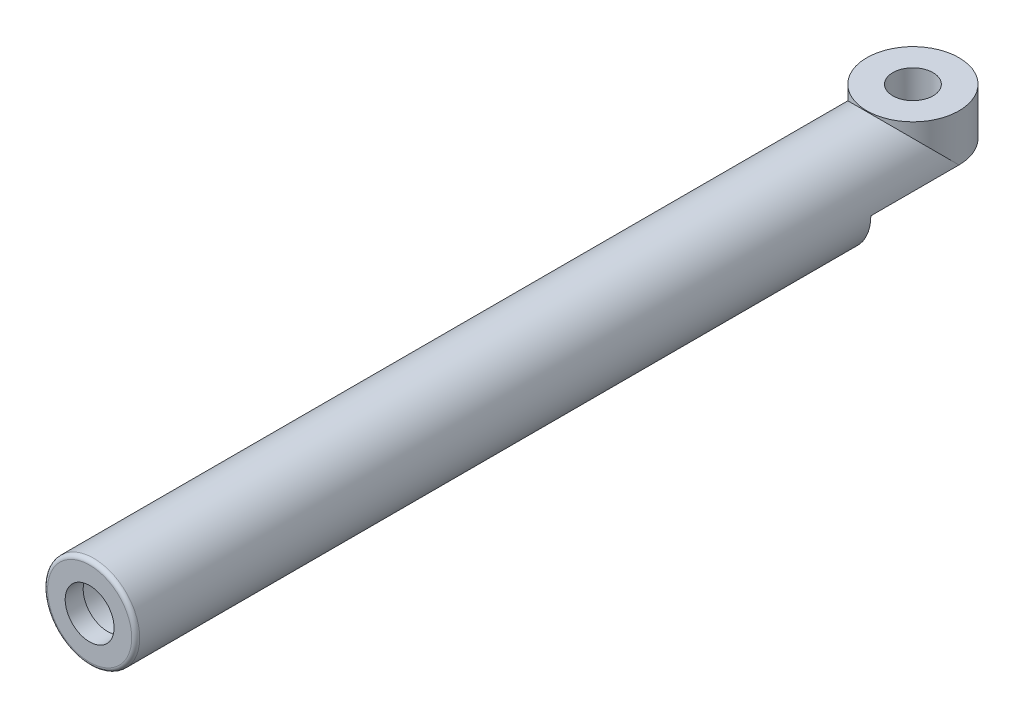
ISO-10303-21;
HEADER;
FILE_DESCRIPTION(('STEP AP214'),'2;1');
FILE_NAME('part.step','',(''),(''),'','','');
FILE_SCHEMA(('AUTOMOTIVE_DESIGN { 1 0 10303 214 1 1 1 1 }'));
ENDSEC;
DATA;
#1=APPLICATION_CONTEXT('core data for automotive mechanical design processes');
#2=APPLICATION_PROTOCOL_DEFINITION('international standard','automotive_design',2000,#1);
#3=PRODUCT_CONTEXT('',#1,'mechanical');
#4=PRODUCT('Part','Part','',(#3));
#5=PRODUCT_RELATED_PRODUCT_CATEGORY('part','',(#4));
#6=PRODUCT_DEFINITION_FORMATION('','',#4);
#7=PRODUCT_DEFINITION_CONTEXT('part definition',#1,'design');
#8=PRODUCT_DEFINITION('design','',#6,#7);
#9=PRODUCT_DEFINITION_SHAPE('','',#8);
#10=(LENGTH_UNIT() NAMED_UNIT(*) SI_UNIT(.MILLI.,.METRE.));
#11=(NAMED_UNIT(*) PLANE_ANGLE_UNIT() SI_UNIT($,.RADIAN.));
#12=(NAMED_UNIT(*) SI_UNIT($,.STERADIAN.) SOLID_ANGLE_UNIT());
#13=UNCERTAINTY_MEASURE_WITH_UNIT(LENGTH_MEASURE(1.E-05),#10,'distance_accuracy_value','');
#14=(GEOMETRIC_REPRESENTATION_CONTEXT(3) GLOBAL_UNCERTAINTY_ASSIGNED_CONTEXT((#13)) GLOBAL_UNIT_ASSIGNED_CONTEXT((#10,
#11,#12)) REPRESENTATION_CONTEXT('',''));
#15=CARTESIAN_POINT('',(0.,0.,0.));
#16=DIRECTION('',(0.,0.,1.));
#17=DIRECTION('',(1.,0.,0.));
#18=AXIS2_PLACEMENT_3D('',#15,#16,#17);
#19=CARTESIAN_POINT('',(0.,0.,1100.));
#20=DIRECTION('',(0.,0.,-1.));
#21=DIRECTION('',(-1.,0.,0.));
#22=AXIS2_PLACEMENT_3D('',#19,#20,#21);
#23=CYLINDRICAL_SURFACE('',#22,115.);
#24=CARTESIAN_POINT('',(0.,0.,1090.));
#25=DIRECTION('',(0.,0.,1.));
#26=DIRECTION('',(1.,0.,0.));
#27=AXIS2_PLACEMENT_3D('',#24,#25,#26);
#28=CIRCLE('',#27,115.);
#29=CARTESIAN_POINT('',(115.,0.,1090.));
#30=VERTEX_POINT('',#29);
#31=EDGE_CURVE('E11',#30,#30,#28,.F.);
#32=ORIENTED_EDGE('',*,*,#31,.T.);
#33=EDGE_LOOP('',(#32));
#34=FACE_BOUND('',#33,.T.);
#35=DIRECTION('',(0.,0.,-1.));
#36=VECTOR('',#35,1.);
#37=CARTESIAN_POINT('',(115.,0.,-1100.));
#38=LINE('',#37,#36);
#39=CARTESIAN_POINT('',(115.,0.,-735.));
#40=VERTEX_POINT('',#39);
#41=CARTESIAN_POINT('',(115.,0.,-955.));
#42=VERTEX_POINT('',#41);
#43=EDGE_CURVE('E65',#40,#42,#38,.T.);
#44=ORIENTED_EDGE('',*,*,#43,.T.);
#45=CARTESIAN_POINT('',(0.,0.,-955.));
#46=DIRECTION('',(0.,0.707106781186547,-0.707106781186547));
#47=DIRECTION('',(0.,-0.707106781186547,-0.707106781186547));
#48=AXIS2_PLACEMENT_3D('',#45,#46,#47);
#49=ELLIPSE('',#48,162.634559672906,115.);
#50=CARTESIAN_POINT('',(-115.,0.,-955.));
#51=VERTEX_POINT('',#50);
#52=EDGE_CURVE('E79',#42,#51,#49,.F.);
#53=ORIENTED_EDGE('',*,*,#52,.T.);
#54=DIRECTION('',(0.,0.,1.));
#55=VECTOR('',#54,1.);
#56=CARTESIAN_POINT('',(-115.,0.,-1100.));
#57=LINE('',#56,#55);
#58=CARTESIAN_POINT('',(-115.,0.,-735.));
#59=VERTEX_POINT('',#58);
#60=EDGE_CURVE('E68',#51,#59,#57,.T.);
#61=ORIENTED_EDGE('',*,*,#60,.T.);
#62=CARTESIAN_POINT('',(0.,0.,-735.));
#63=DIRECTION('',(0.,0.,1.));
#64=DIRECTION('',(1.,0.,0.));
#65=AXIS2_PLACEMENT_3D('',#62,#63,#64);
#66=CIRCLE('',#65,115.);
#67=EDGE_CURVE('E83',#59,#40,#66,.T.);
#68=ORIENTED_EDGE('',*,*,#67,.T.);
#69=EDGE_LOOP('',(#44,#53,#61,#68));
#70=FACE_BOUND('',#69,.T.);
#71=ADVANCED_FACE('F43',(#34,#70),#23,.T.);
#72=CARTESIAN_POINT('',(0.,-1100.,-955.));
#73=DIRECTION('',(0.,1.,0.));
#74=DIRECTION('',(0.,0.,1.));
#75=AXIS2_PLACEMENT_3D('',#72,#73,#74);
#76=CYLINDRICAL_SURFACE('',#75,50.25);
#77=CARTESIAN_POINT('',(0.,0.,-955.));
#78=DIRECTION('',(0.,1.,0.));
#79=DIRECTION('',(0.,0.,1.));
#80=AXIS2_PLACEMENT_3D('',#77,#78,#79);
#81=CIRCLE('',#80,50.25);
#82=CARTESIAN_POINT('',(0.,0.,-904.75));
#83=VERTEX_POINT('',#82);
#84=EDGE_CURVE('E88',#83,#83,#81,.F.);
#85=ORIENTED_EDGE('',*,*,#84,.T.);
#86=EDGE_LOOP('',(#85));
#87=FACE_BOUND('',#86,.T.);
#88=CARTESIAN_POINT('',(0.,117.,-955.));
#89=DIRECTION('',(0.,-1.,0.));
#90=DIRECTION('',(0.,0.,-1.));
#91=AXIS2_PLACEMENT_3D('',#88,#89,#90);
#92=CIRCLE('',#91,50.25);
#93=CARTESIAN_POINT('',(0.,117.,-1005.25));
#94=VERTEX_POINT('',#93);
#95=EDGE_CURVE('E110',#94,#94,#92,.T.);
#96=ORIENTED_EDGE('',*,*,#95,.F.);
#97=EDGE_LOOP('',(#96));
#98=FACE_BOUND('',#97,.T.);
#99=ADVANCED_FACE('F112',(#87,#98),#76,.F.);
#100=CARTESIAN_POINT('',(0.,0.,0.));
#101=DIRECTION('',(0.,1.,0.));
#102=DIRECTION('',(0.,0.,1.));
#103=AXIS2_PLACEMENT_3D('',#100,#101,#102);
#104=PLANE('',#103);
#105=ORIENTED_EDGE('',*,*,#60,.F.);
#106=CARTESIAN_POINT('',(0.,0.,-955.));
#107=DIRECTION('',(0.,1.,0.));
#108=DIRECTION('',(0.,0.,1.));
#109=AXIS2_PLACEMENT_3D('',#106,#107,#108);
#110=CIRCLE('',#109,115.);
#111=EDGE_CURVE('E59',#42,#51,#110,.T.);
#112=ORIENTED_EDGE('',*,*,#111,.F.);
#113=ORIENTED_EDGE('',*,*,#43,.F.);
#114=DIRECTION('',(1.,0.,0.));
#115=VECTOR('',#114,1.);
#116=CARTESIAN_POINT('',(-115.,0.,-735.));
#117=LINE('',#116,#115);
#118=EDGE_CURVE('E71',#59,#40,#117,.T.);
#119=ORIENTED_EDGE('',*,*,#118,.F.);
#120=EDGE_LOOP('',(#105,#112,#113,#119));
#121=FACE_BOUND('',#120,.T.);
#122=ORIENTED_EDGE('',*,*,#84,.F.);
#123=EDGE_LOOP('',(#122));
#124=FACE_BOUND('',#123,.T.);
#125=ADVANCED_FACE('F69',(#121,#124),#104,.F.);
#126=CARTESIAN_POINT('',(0.,0.,1100.));
#127=DIRECTION('',(0.,0.,1.));
#128=DIRECTION('',(1.,0.,0.));
#129=AXIS2_PLACEMENT_3D('',#126,#127,#128);
#130=PLANE('',#129);
#131=CARTESIAN_POINT('',(0.,0.,1100.));
#132=DIRECTION('',(0.,0.,1.));
#133=DIRECTION('',(1.,0.,0.));
#134=AXIS2_PLACEMENT_3D('',#131,#132,#133);
#135=CIRCLE('',#134,105.);
#136=CARTESIAN_POINT('',(105.,0.,1100.));
#137=VERTEX_POINT('',#136);
#138=EDGE_CURVE('E51',#137,#137,#135,.T.);
#139=ORIENTED_EDGE('',*,*,#138,.T.);
#140=EDGE_LOOP('',(#139));
#141=FACE_BOUND('',#140,.T.);
#142=CARTESIAN_POINT('',(0.,0.,1100.));
#143=DIRECTION('',(0.,0.,1.));
#144=DIRECTION('',(1.,0.,0.));
#145=AXIS2_PLACEMENT_3D('',#142,#143,#144);
#146=CIRCLE('',#145,61.);
#147=CARTESIAN_POINT('',(61.,0.,1100.));
#148=VERTEX_POINT('',#147);
#149=EDGE_CURVE('E77',#148,#148,#146,.T.);
#150=ORIENTED_EDGE('',*,*,#149,.F.);
#151=EDGE_LOOP('',(#150));
#152=FACE_BOUND('',#151,.T.);
#153=ADVANCED_FACE('F125',(#141,#152),#130,.T.);
#154=CARTESIAN_POINT('',(-115.,-2200.,-735.));
#155=DIRECTION('',(0.,0.,1.));
#156=DIRECTION('',(1.,0.,0.));
#157=AXIS2_PLACEMENT_3D('',#154,#155,#156);
#158=PLANE('',#157);
#159=ORIENTED_EDGE('',*,*,#118,.T.);
#160=ORIENTED_EDGE('',*,*,#67,.F.);
#161=EDGE_LOOP('',(#159,#160));
#162=FACE_BOUND('',#161,.T.);
#163=ADVANCED_FACE('F129',(#162),#158,.F.);
#164=CARTESIAN_POINT('',(0.,0.,1100.));
#165=DIRECTION('',(0.,0.,1.));
#166=DIRECTION('',(1.,0.,0.));
#167=AXIS2_PLACEMENT_3D('',#164,#165,#166);
#168=CYLINDRICAL_SURFACE('',#167,61.);
#169=CARTESIAN_POINT('',(0.,0.,1055.10287079519));
#170=DIRECTION('',(0.,0.,1.));
#171=DIRECTION('',(1.,0.,0.));
#172=AXIS2_PLACEMENT_3D('',#169,#170,#171);
#173=CIRCLE('',#172,61.);
#174=CARTESIAN_POINT('',(61.,0.,1055.10287079519));
#175=VERTEX_POINT('',#174);
#176=EDGE_CURVE('E97',#175,#175,#173,.T.);
#177=ORIENTED_EDGE('',*,*,#176,.F.);
#178=EDGE_LOOP('',(#177));
#179=FACE_BOUND('',#178,.T.);
#180=ORIENTED_EDGE('',*,*,#149,.T.);
#181=EDGE_LOOP('',(#180));
#182=FACE_BOUND('',#181,.T.);
#183=ADVANCED_FACE('F134',(#179,#182),#168,.F.);
#184=CARTESIAN_POINT('',(61.,0.,1055.10287079519));
#185=DIRECTION('',(0.,0.,1.));
#186=DIRECTION('',(1.,0.,0.));
#187=AXIS2_PLACEMENT_3D('',#184,#185,#186);
#188=PLANE('',#187);
#189=CARTESIAN_POINT('',(0.,0.,1055.10287079519));
#190=DIRECTION('',(0.,0.,1.));
#191=DIRECTION('',(1.,0.,0.));
#192=AXIS2_PLACEMENT_3D('',#189,#190,#191);
#193=CIRCLE('',#192,81.);
#194=CARTESIAN_POINT('',(81.,0.,1055.10287079519));
#195=VERTEX_POINT('',#194);
#196=EDGE_CURVE('E99',#195,#195,#193,.T.);
#197=ORIENTED_EDGE('',*,*,#196,.F.);
#198=EDGE_LOOP('',(#197));
#199=FACE_BOUND('',#198,.T.);
#200=ORIENTED_EDGE('',*,*,#176,.T.);
#201=EDGE_LOOP('',(#200));
#202=FACE_BOUND('',#201,.T.);
#203=ADVANCED_FACE('F145',(#199,#202),#188,.F.);
#204=CARTESIAN_POINT('',(0.,0.,1100.));
#205=DIRECTION('',(0.,0.,1.));
#206=DIRECTION('',(1.,0.,0.));
#207=AXIS2_PLACEMENT_3D('',#204,#205,#206);
#208=CYLINDRICAL_SURFACE('',#207,81.);
#209=CARTESIAN_POINT('',(0.,0.,-685.));
#210=DIRECTION('',(0.,0.,1.));
#211=DIRECTION('',(1.,0.,0.));
#212=AXIS2_PLACEMENT_3D('',#209,#210,#211);
#213=CIRCLE('',#212,81.);
#214=CARTESIAN_POINT('',(81.,0.,-685.));
#215=VERTEX_POINT('',#214);
#216=EDGE_CURVE('E82',#215,#215,#213,.T.);
#217=ORIENTED_EDGE('',*,*,#216,.F.);
#218=EDGE_LOOP('',(#217));
#219=FACE_BOUND('',#218,.T.);
#220=ORIENTED_EDGE('',*,*,#196,.T.);
#221=EDGE_LOOP('',(#220));
#222=FACE_BOUND('',#221,.T.);
#223=ADVANCED_FACE('F149',(#219,#222),#208,.F.);
#224=CARTESIAN_POINT('',(81.,0.,-685.));
#225=DIRECTION('',(0.,0.,-1.));
#226=DIRECTION('',(-1.,0.,0.));
#227=AXIS2_PLACEMENT_3D('',#224,#225,#226);
#228=PLANE('',#227);
#229=ORIENTED_EDGE('',*,*,#216,.T.);
#230=EDGE_LOOP('',(#229));
#231=FACE_BOUND('',#230,.T.);
#232=ADVANCED_FACE('F154',(#231),#228,.F.);
#233=CARTESIAN_POINT('',(0.,117.,-955.));
#234=DIRECTION('',(0.,-1.,0.));
#235=DIRECTION('',(0.,0.,-1.));
#236=AXIS2_PLACEMENT_3D('',#233,#234,#235);
#237=CYLINDRICAL_SURFACE('',#236,115.);
#238=CARTESIAN_POINT('',(0.,117.,-955.));
#239=DIRECTION('',(0.,-1.,0.));
#240=DIRECTION('',(0.,0.,-1.));
#241=AXIS2_PLACEMENT_3D('',#238,#239,#240);
#242=CIRCLE('',#241,115.);
#243=CARTESIAN_POINT('',(0.,117.,-1070.));
#244=VERTEX_POINT('',#243);
#245=EDGE_CURVE('E85',#244,#244,#242,.T.);
#246=ORIENTED_EDGE('',*,*,#245,.T.);
#247=EDGE_LOOP('',(#246));
#248=FACE_BOUND('',#247,.T.);
#249=ORIENTED_EDGE('',*,*,#52,.F.);
#250=ORIENTED_EDGE('',*,*,#111,.T.);
#251=EDGE_LOOP('',(#249,#250));
#252=FACE_BOUND('',#251,.T.);
#253=ADVANCED_FACE('F81',(#248,#252),#237,.T.);
#254=CARTESIAN_POINT('',(0.,117.,-955.));
#255=DIRECTION('',(0.,-1.,0.));
#256=DIRECTION('',(0.,0.,-1.));
#257=AXIS2_PLACEMENT_3D('',#254,#255,#256);
#258=PLANE('',#257);
#259=ORIENTED_EDGE('',*,*,#95,.T.);
#260=EDGE_LOOP('',(#259));
#261=FACE_BOUND('',#260,.T.);
#262=ORIENTED_EDGE('',*,*,#245,.F.);
#263=EDGE_LOOP('',(#262));
#264=FACE_BOUND('',#263,.T.);
#265=ADVANCED_FACE('F111',(#261,#264),#258,.F.);
#266=CARTESIAN_POINT('',(0.,0.,1090.));
#267=DIRECTION('',(0.,0.,1.));
#268=DIRECTION('',(1.,0.,0.));
#269=AXIS2_PLACEMENT_3D('',#266,#267,#268);
#270=TOROIDAL_SURFACE('',#269,105.,10.);
#271=ORIENTED_EDGE('',*,*,#31,.F.);
#272=EDGE_LOOP('',(#271));
#273=FACE_BOUND('',#272,.T.);
#274=ORIENTED_EDGE('',*,*,#138,.F.);
#275=EDGE_LOOP('',(#274));
#276=FACE_BOUND('',#275,.T.);
#277=ADVANCED_FACE('F44',(#273,#276),#270,.T.);
#278=CLOSED_SHELL('',(#71,#99,#125,#153,#163,#183,#203,#223,#232,#253,#265,#277));
#279=MANIFOLD_SOLID_BREP('B2',#278);
#280=ADVANCED_BREP_SHAPE_REPRESENTATION('',(#18,#279),#14);
#281=SHAPE_DEFINITION_REPRESENTATION(#9,#280);
ENDSEC;
END-ISO-10303-21;
